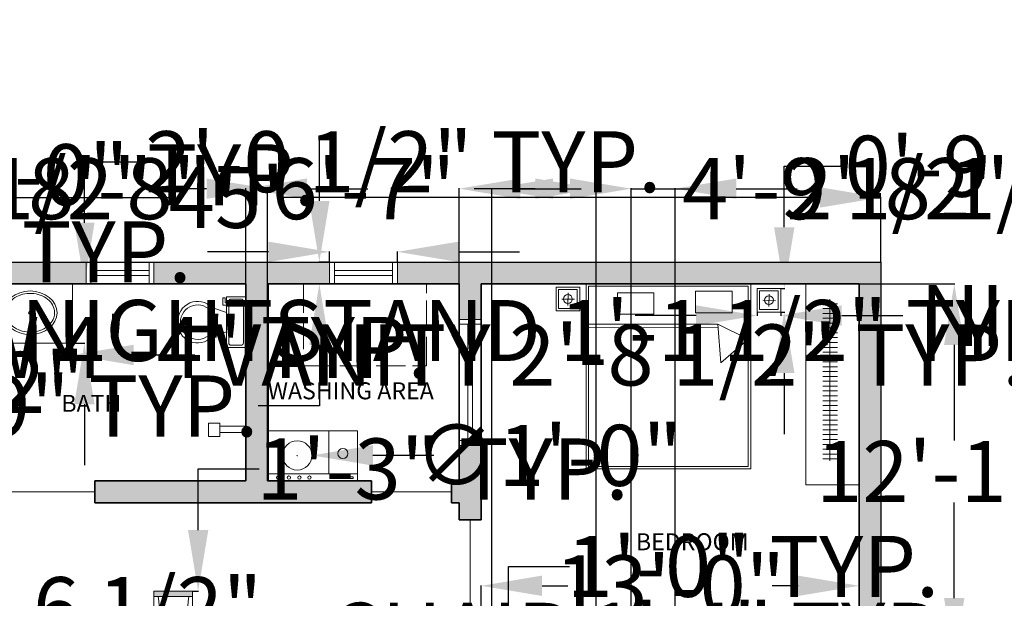
# Model space of a CAD drawing. Units: inches. Extents: x 29 to 6336, y 3 to 2592.
# Tile 7 of 8: x 5531 to 5938, y 2354 to 2592. Entities that reach past the tile are written whole.
import ezdxf

# ---------------------------------------------------------------- set-up
doc = ezdxf.new("R2010")
doc.units = ezdxf.units.IN
doc.header["$MEASUREMENT"] = 0
doc.linetypes.add('ACAD_ISO02W100', pattern=[15, 12, -3])
for name, color, linetype, lineweight in [('A-ANNO-DIMS', 2, 'Continuous', 18), ('A-AREA-IDEN', 7, 'Continuous', 18), ('A-DOOR', 4, 'Continuous', 18), ('A-EQPM', 9, 'Continuous', 18), ('A-EQPM-OVHD', 9, 'ACAD_ISO02W100', 13), ('A-FLOR-CASE', 8, 'Continuous', 18), ('A-FLOR-FIXT', 8, 'Continuous', 18), ('A-FURN', 8, 'Continuous', 18), ('A-GLAZ', 116, 'Continuous', 18), ('A-WALL', 7, 'Continuous', 35), ('A-WALL-PATT', 242, 'Continuous', 13), ('C-PROP', 7, 'Continuous', 25)]:
    doc.layers.add(name, color=color, linetype=linetype, lineweight=lineweight)
doc.styles.get("Standard").update_dxf_attribs({"font": 'arial.ttf'})
doc.dimstyles.get("Standard").update_dxf_attribs({"dimtxt": 25.18, "dimasz": 25.18, "dimexe": 0.18, "dimexo": 0.0625, "dimgap": 0.09, "dimtad": 0, "dimtih": 1, "dimtoh": 1, "dimdec": 0, "dimzin": 0, "dimdsep": 46, "dimlunit": 3, "dimtxsty": 'Standard', "dimcen": 0.09, "dimadec": 0, "dimazin": 0, "dimtfac": 1, "dimtdec": 0, "dimtofl": 0, "dimtmove": 0, "dimatfit": 3, "dimfxl": 1, "dimtolj": 1, "dimtzin": 0, "dimarcsym": 0})

# ---------------------------------------------------------------- blocks, each defined once
blk = doc.blocks.new('*U4')
for p, q in [((9.5, -6), (9.5, -2)), ((-8, -8.5), (-8, -8)), ((-7, -8), (-7, -9.5)), ((-4, -8), (-6, -14)), ((4, -8), (6, -14)), ((-10, -8.5), (-8, -8.5)), ((-10, -9.5), (-10, -8.5)), ((-7, -9.5), (-10, -9.5)), ((4, -14), (-4, -14))]:
    blk.add_line(p, q)
blk.add_lwpolyline([(10.5, -8), (10.5, 0), (-10.5, 0), (-10.5, -8)], close=True)
for points in [[(-9.5, -2), (-9.5, -6)], [(8.5, -1), (-8.5, -1)], [(-8.5, -7), (8.5, -7)]]:
    blk.add_lwpolyline(points)
for centre, radius, start, end in [((-8.625, -1.875), 0.8839, 81.8699, 188.1301), ((8.625, -1.875), 0.8839, 351.8699, 98.1301), ((-8.625, -6.125), 0.8839, 171.869898, 278.1301), ((8.625, -6.125), 0.8839, 261.8699, 8.1301), ((-0.4772, -19.9188), 8.0953, 133.01722, 273.38), ((0.0374, -19.8731), 7.127, 124.50543, 269.7), ((-0.0373, -19.8731), 7.127, 270.3, 55.4946), ((0.4773, -19.9188), 8.0953, 266.62, 46.9828)]:
    blk.add_arc(centre, radius, start, end)
blk = doc.blocks.new('*D5')
at = {"layer": 'A-ANNO-DIMS', "color": 0, "lineweight": -2, "transparency": 16777216}
for p, q in [((5346.66, 2492.39), (5346.66, 2519.15)), ((5371.84, 2518.97), (5594.69, 2518.97)), ((5861.48, 2518.97), (5638.62, 2518.97)), ((5886.66, 2492.39), (5886.66, 2519.15))]:
    blk.add_line(p, q, dxfattribs=at)
at = {"layer": 'A-ANNO-DIMS', "color": 0, "transparency": 16777216}
for points in [[(5371.84, 2523.17), (5371.84, 2514.77), (5346.66, 2518.97)], [(5861.48, 2523.17), (5861.48, 2514.77), (5886.66, 2518.97)]]:
    blk.add_solid(points, dxfattribs=at)
at = {"layer": 'Defpoints', "color": 0, "transparency": 16777216}
for p in [(5886.66, 2518.97), (5346.66, 2492.33), (5886.66, 2492.33)]:
    blk.add_point(p, dxfattribs=at)
at = {"layer": 'A-ANNO-DIMS', "color": 0, "transparency": 16777216, "insert": (5616.66, 2518.97), "char_height": 25.18, "attachment_point": 5}
blk.add_mtext("\\A1;45'", dxfattribs=at)
blk = doc.blocks.new('WIN-48')
for p, q in [((0, 9), (0, 0)), ((2, 9), (2, 0)), ((50, 9), (50, 0)), ((52, 9), (52, 0)), ((2, 5.5), (50, 5.5)), ((2, 3.5), (50, 3.5))]:
    blk.add_line(p, q)
blk = doc.blocks.new('WIN-24')
for p, q in [((0, 9), (0, 0)), ((2, 9), (2, 0)), ((26, 9), (26, 0)), ((28, 9), (28, 0)), ((2, 5.5), (26, 5.5)), ((2, 3.5), (26, 3.5))]:
    blk.add_line(p, q)
blk = doc.blocks.new('CHAIR-DINING')
h = blk.add_hatch(color=256)
h.dxf.hatch_style = 1
h.paths.add_polyline_path([(15.9, 12.75), (15.9, 15.02), (0, 15.02), (0, 12.75)])
for p, q in [((0, 0), (0, 15.02)), ((0, 15.02), (15.9, 15.02)), ((0, 12.75), (15.9, 12.75)), ((15.9, 15.02), (15.9, 0))]:
    blk.add_line(p, q)
for points in [[(1.75, 12.75), (2.84, 7.81), (1.97, 2.88), (1.75, 0)], [(14.44, 12.75), (13.78, 7.03), (13.63, 2.52), (14.44, 0)]]:
    blk.add_open_spline(points, degree=3)
blk = doc.blocks.new('NIGHTSTAND-10X10')
for p, q in [((2.31, 4.87), (7.57, 4.8)), ((4.94, 7.35), (4.88, 2.25))]:
    blk.add_line(p, q)
for points in [[(0, 9.74), (9.74, 9.74), (9.74, 0), (0, 0)], [(1, 8.74), (8.74, 8.74), (8.74, 1), (1, 1)]]:
    blk.add_lwpolyline(points, close=True)
blk.add_circle((4.87, 4.87), 1.82)
blk = doc.blocks.new('BASIN-VANITY')
for p, q in [((32.36, 0), (32.36, 24.47)), ((0, 0), (32.36, 0))]:
    blk.add_line(p, q)
blk.add_circle((14.85, 12.56), 0.667)
blk.add_ellipse((14.85, 12.56), major_axis=(11.1, 0), ratio=0.808824)
blk.add_open_spline([(24.95, 12.56), (24.95, 13.21), (24.85, 13.86), (24.35, 15.41), (23.86, 16.28), (22.49, 17.85), (21.62, 18.55), (19.61, 19.66), (18.47, 20.07), (16.07, 20.54), (14.82, 20.6), (12.37, 20.35), (11.18, 20.05), (9.01, 19.14), (8.04, 18.52), (6.44, 17.08), (5.81, 16.25), (4.97, 14.49), (4.75, 13.56), (4.73, 11.7), (4.93, 10.77), (5.73, 9), (6.33, 8.16), (7.89, 6.69), (8.85, 6.07), (10.99, 5.12), (12.18, 4.8), (14.62, 4.52), (15.88, 4.56), (18.29, 4.99), (19.44, 5.38), (21.47, 6.46), (22.36, 7.14), (23.77, 8.7), (24.29, 9.57), (24.83, 11.15), (24.95, 11.85), (24.95, 12.56)], degree=3, knots=[0, 0, 0, 0, 0.253102, 0.253102, 0.612978, 0.612978, 0.972853, 0.972853, 1.332728, 1.332728, 1.692603, 1.692603, 2.052478, 2.052478, 2.412354, 2.412354, 2.772229, 2.772229, 3.132104, 3.132104, 3.491979, 3.491979, 3.851854, 3.851854, 4.21173, 4.21173, 4.571605, 4.571605, 4.93148, 4.93148, 5.291355, 5.291355, 5.651231, 5.651231, 6.011106, 6.011106, 6.283185, 6.283185, 6.283185, 6.283185])
blk = doc.blocks.new('*D20')
at = {"layer": 'A-ANNO-DIMS', "color": 0, "lineweight": -2, "transparency": 16777216}
for p, q in [((5586.64, 2341.55), (5586.64, 2339.04)), ((5602.54, 2341.55), (5602.54, 2339.04)), ((5561.46, 2339.22), (5536.28, 2339.22)), ((5627.72, 2339.22), (5652.9, 2339.22))]:
    blk.add_line(p, q, dxfattribs=at)
at = {"layer": 'A-ANNO-DIMS', "color": 0, "transparency": 16777216}
for points in [[(5561.46, 2343.42), (5561.46, 2335.03), (5586.64, 2339.22)], [(5627.72, 2343.42), (5627.72, 2335.03), (5602.54, 2339.22)]]:
    blk.add_solid(points, dxfattribs=at)
at = {"layer": 'Defpoints', "color": 0, "transparency": 16777216}
for p in [(5586.64, 2341.61), (5602.54, 2341.61), (5602.54, 2339.22)]:
    blk.add_point(p, dxfattribs=at)
at = {"layer": 'A-ANNO-DIMS', "color": 0, "transparency": 16777216, "insert": (5789.2, 2339.22), "char_height": 25.18, "attachment_point": 5}
blk.add_mtext('\\A1;CHAIR 1\'-4" TYP.', dxfattribs=at)
blk = doc.blocks.new('*D21')
at = {"layer": 'A-ANNO-DIMS', "color": 0, "lineweight": -2, "transparency": 16777216}
for p, q in [((5604.93, 2381.81), (5604.93, 2406.99)), ((5604.93, 2406.99), (5630.11, 2406.99)), ((5602.6, 2356.63), (5605.11, 2356.63)), ((5602.6, 2341.61), (5605.11, 2341.61)), ((5604.93, 2316.43), (5604.93, 2291.25))]:
    blk.add_line(p, q, dxfattribs=at)
at = {"layer": 'A-ANNO-DIMS', "color": 0, "transparency": 16777216}
for points in [[(5600.73, 2381.81), (5609.12, 2381.81), (5604.93, 2356.63)], [(5600.73, 2316.43), (5609.12, 2316.43), (5604.93, 2341.61)]]:
    blk.add_solid(points, dxfattribs=at)
at = {"layer": 'Defpoints', "color": 0, "transparency": 16777216}
for p in [(5602.54, 2356.63), (5604.93, 2356.63), (5602.54, 2341.61)]:
    blk.add_point(p, dxfattribs=at)
at = {"layer": 'A-ANNO-DIMS', "color": 0, "transparency": 16777216, "insert": (5705.75, 2406.99), "char_height": 25.18, "attachment_point": 5}
blk.add_mtext('\\A1;1\'-3" TYP.', dxfattribs=at)
blk = doc.blocks.new('*D22')
at = {"layer": 'A-ANNO-DIMS', "color": 0, "lineweight": -2, "transparency": 16777216}
for p, q in [((5363.46, 2431.95), (5363.46, 2457.13)), ((5363.46, 2457.13), (5388.64, 2457.13)), ((5355.72, 2431.95), (5363.64, 2431.95)), ((5363.46, 2405.13), (5363.46, 2406.77)), ((5355.72, 2379.95), (5363.64, 2379.95))]:
    blk.add_line(p, q, dxfattribs=at)
at = {"layer": 'A-ANNO-DIMS', "color": 0, "transparency": 16777216}
for points in [[(5359.26, 2406.77), (5367.65, 2406.77), (5363.46, 2431.95)], [(5359.26, 2405.13), (5367.65, 2405.13), (5363.46, 2379.95)]]:
    blk.add_solid(points, dxfattribs=at)
at = {"layer": 'Defpoints', "color": 0, "transparency": 16777216}
for p in [(5355.66, 2431.95), (5363.46, 2431.95), (5355.66, 2379.95)]:
    blk.add_point(p, dxfattribs=at)
at = {"layer": 'A-ANNO-DIMS', "color": 0, "transparency": 16777216, "insert": (5548.04, 2457.13), "char_height": 25.18, "attachment_point": 5}
blk.add_mtext('\\A1;WINDOW 4\'-4" TYP.', dxfattribs=at)
blk = doc.blocks.new('*D26')
at = {"layer": 'A-ANNO-DIMS', "color": 0, "lineweight": -2, "transparency": 16777216}
for p, q in [((5633.95, 2496.53), (5608.77, 2496.53)), ((5659.13, 2492.39), (5659.13, 2496.71)), ((5687.13, 2492.39), (5687.13, 2496.71)), ((5712.31, 2496.53), (5737.49, 2496.53))]:
    blk.add_line(p, q, dxfattribs=at)
at = {"layer": 'A-ANNO-DIMS', "color": 0, "transparency": 16777216}
for points in [[(5633.95, 2500.73), (5633.95, 2492.33), (5659.13, 2496.53)], [(5712.31, 2500.73), (5712.31, 2492.33), (5687.13, 2496.53)]]:
    blk.add_solid(points, dxfattribs=at)
at = {"layer": 'Defpoints', "color": 0, "transparency": 16777216}
for p in [(5659.13, 2496.53), (5659.13, 2492.33), (5687.13, 2492.33)]:
    blk.add_point(p, dxfattribs=at)
at = {"layer": 'A-ANNO-DIMS', "color": 0, "transparency": 16777216, "insert": (5449.36, 2496.53), "char_height": 25.18, "attachment_point": 5}
blk.add_mtext('\\A1;WINDOW 2\'-4" TYP.', dxfattribs=at)
blk = doc.blocks.new('*D27')
at = {"layer": 'A-ANNO-DIMS', "color": 0, "lineweight": -2, "transparency": 16777216}
for p, q in [((5654.93, 2517.51), (5654.93, 2542.69)), ((5659.07, 2492.33), (5654.75, 2492.33)), ((5659.07, 2483.33), (5654.75, 2483.33)), ((5654.93, 2458.15), (5654.93, 2432.97)), ((5654.93, 2432.97), (5629.75, 2432.97))]:
    blk.add_line(p, q, dxfattribs=at)
at = {"layer": 'A-ANNO-DIMS', "color": 0, "transparency": 16777216}
for points in [[(5650.73, 2517.51), (5659.12, 2517.51), (5654.93, 2492.33)], [(5650.73, 2458.15), (5659.12, 2458.15), (5654.93, 2483.33)]]:
    blk.add_solid(points, dxfattribs=at)
at = {"layer": 'Defpoints', "color": 0, "transparency": 16777216}
for p in [(5659.13, 2492.33), (5654.93, 2483.33), (5659.13, 2483.33)]:
    blk.add_point(p, dxfattribs=at)
at = {"layer": 'A-ANNO-DIMS', "color": 0, "transparency": 16777216, "insert": (5552.92, 2432.97), "char_height": 25.18, "attachment_point": 5}
blk.add_mtext('\\A1;0\'-9" TYP.', dxfattribs=at)
blk = doc.blocks.new('*D30')
at = {"layer": 'A-ANNO-DIMS', "color": 0, "lineweight": -2, "transparency": 16777216}
for p, q in [((5810.39, 2470.26), (5785.21, 2470.26)), ((5835.57, 2471.66), (5835.57, 2470.08)), ((5845.31, 2471.66), (5845.31, 2470.08)), ((5870.49, 2470.26), (5895.67, 2470.26))]:
    blk.add_line(p, q, dxfattribs=at)
at = {"layer": 'A-ANNO-DIMS', "color": 0, "transparency": 16777216}
for points in [[(5810.39, 2474.46), (5810.39, 2466.06), (5835.57, 2470.26)], [(5870.49, 2474.46), (5870.49, 2466.06), (5845.31, 2470.26)]]:
    blk.add_solid(points, dxfattribs=at)
at = {"layer": 'Defpoints', "color": 0, "transparency": 16777216}
for p in [(5835.57, 2471.72), (5845.31, 2471.72), (5845.31, 2470.26)]:
    blk.add_point(p, dxfattribs=at)
at = {"layer": 'A-ANNO-DIMS', "color": 0, "transparency": 16777216, "insert": (6120.44, 2470.26), "char_height": 25.18, "attachment_point": 5}
blk.add_mtext('\\A1;NIGHTSTAND 0\'-9 1/2" TYP.', dxfattribs=at)
blk = doc.blocks.new('*D31')
at = {"layer": 'A-ANNO-DIMS', "color": 0, "lineweight": -2, "transparency": 16777216}
for p, q in [((5846.78, 2506.64), (5846.78, 2531.82)), ((5846.78, 2531.82), (5871.96, 2531.82)), ((5845.38, 2481.46), (5846.96, 2481.46)), ((5845.38, 2471.72), (5846.96, 2471.72)), ((5846.78, 2446.54), (5846.78, 2421.36))]:
    blk.add_line(p, q, dxfattribs=at)
at = {"layer": 'A-ANNO-DIMS', "color": 0, "transparency": 16777216}
for points in [[(5842.58, 2506.64), (5850.97, 2506.64), (5846.78, 2481.46)], [(5842.58, 2446.54), (5850.97, 2446.54), (5846.78, 2471.72)]]:
    blk.add_solid(points, dxfattribs=at)
at = {"layer": 'Defpoints', "color": 0, "transparency": 16777216}
for p in [(5845.31, 2481.46), (5846.78, 2481.46), (5845.31, 2471.72)]:
    blk.add_point(p, dxfattribs=at)
at = {"layer": 'A-ANNO-DIMS', "color": 0, "transparency": 16777216, "insert": (5978.13, 2531.82), "char_height": 25.18, "attachment_point": 5}
blk.add_mtext('\\A1;0\'-9 1/2" TYP.', dxfattribs=at)
blk = doc.blocks.new('*D32')
at = {"layer": 'A-ANNO-DIMS', "color": 0, "lineweight": -2, "transparency": 16777216}
for p, q in [((5709.84, 2318.47), (5684.66, 2318.47)), ((5735.02, 2316.52), (5735.02, 2318.65)), ((5748.43, 2316.52), (5748.43, 2318.65)), ((5773.61, 2318.47), (5798.79, 2318.47))]:
    blk.add_line(p, q, dxfattribs=at)
at = {"layer": 'A-ANNO-DIMS', "color": 0, "transparency": 16777216}
for points in [[(5709.84, 2322.67), (5709.84, 2314.27), (5735.02, 2318.47)], [(5773.61, 2322.67), (5773.61, 2314.27), (5748.43, 2318.47)]]:
    blk.add_solid(points, dxfattribs=at)
at = {"layer": 'Defpoints', "color": 0, "transparency": 16777216}
for p in [(5735.02, 2316.46), (5748.43, 2318.47), (5748.43, 2316.46)]:
    blk.add_point(p, dxfattribs=at)
at = {"layer": 'A-ANNO-DIMS', "color": 0, "transparency": 16777216, "insert": (6023.56, 2318.47), "char_height": 25.18, "attachment_point": 5}
blk.add_mtext('\\A1;NIGHTSTAND 1\'-1 1/2" TYP.', dxfattribs=at)
blk = doc.blocks.new('*D33')
at = {"layer": 'A-ANNO-DIMS', "color": 0, "lineweight": -2, "transparency": 16777216}
for p, q in [((5733.01, 2341.64), (5733.01, 2366.82)), ((5733.01, 2366.82), (5758.19, 2366.82)), ((5734.96, 2316.46), (5732.83, 2316.46)), ((5734.96, 2304.36), (5732.83, 2304.36)), ((5733.01, 2279.18), (5733.01, 2254))]:
    blk.add_line(p, q, dxfattribs=at)
at = {"layer": 'A-ANNO-DIMS', "color": 0, "transparency": 16777216}
for points in [[(5728.81, 2341.64), (5737.21, 2341.64), (5733.01, 2316.46)], [(5728.81, 2279.18), (5737.21, 2279.18), (5733.01, 2304.36)]]:
    blk.add_solid(points, dxfattribs=at)
at = {"layer": 'Defpoints', "color": 0, "transparency": 16777216}
for p in [(5733.01, 2316.46), (5735.02, 2316.46), (5735.02, 2304.36)]:
    blk.add_point(p, dxfattribs=at)
at = {"layer": 'A-ANNO-DIMS', "color": 0, "transparency": 16777216, "insert": (5833.84, 2366.82), "char_height": 25.18, "attachment_point": 5}
blk.add_mtext('\\A1;1\'-0" TYP.', dxfattribs=at)
blk = doc.blocks.new('*D36')
at = {"layer": 'A-ANNO-DIMS', "color": 0, "lineweight": -2, "transparency": 16777216}
for p, q in [((5520.77, 2458.79), (5520.77, 2453.82)), ((5553.13, 2458.79), (5553.13, 2453.82)), ((5495.59, 2454), (5470.41, 2454)), ((5578.31, 2454), (5603.49, 2454))]:
    blk.add_line(p, q, dxfattribs=at)
at = {"layer": 'A-ANNO-DIMS', "color": 0, "transparency": 16777216}
for points in [[(5495.59, 2458.2), (5495.59, 2449.81), (5520.77, 2454)], [(5578.31, 2458.2), (5578.31, 2449.81), (5553.13, 2454)]]:
    blk.add_solid(points, dxfattribs=at)
at = {"layer": 'Defpoints', "color": 0, "transparency": 16777216}
for p in [(5520.77, 2458.86), (5553.13, 2458.86), (5553.13, 2454)]:
    blk.add_point(p, dxfattribs=at)
at = {"layer": 'A-ANNO-DIMS', "color": 0, "transparency": 16777216, "insert": (5778.73, 2454), "char_height": 25.18, "attachment_point": 5}
blk.add_mtext('\\A1;VANITY 2\'-8 1/2" TYP.', dxfattribs=at)
blk = doc.blocks.new('*D37')
at = {"layer": 'A-ANNO-DIMS', "color": 0, "lineweight": -2, "transparency": 16777216}
for p, q in [((5557.99, 2508.51), (5557.99, 2533.69)), ((5557.99, 2533.69), (5583.17, 2533.69)), ((5553.2, 2483.33), (5558.17, 2483.33)), ((5553.2, 2458.86), (5558.17, 2458.86)), ((5557.99, 2433.68), (5557.99, 2408.5))]:
    blk.add_line(p, q, dxfattribs=at)
at = {"layer": 'A-ANNO-DIMS', "color": 0, "transparency": 16777216}
for points in [[(5553.79, 2508.51), (5562.18, 2508.51), (5557.99, 2483.33)], [(5553.79, 2433.68), (5562.18, 2433.68), (5557.99, 2458.86)]]:
    blk.add_solid(points, dxfattribs=at)
at = {"layer": 'Defpoints', "color": 0, "transparency": 16777216}
for p in [(5553.13, 2483.33), (5557.99, 2483.33), (5553.13, 2458.86)]:
    blk.add_point(p, dxfattribs=at)
at = {"layer": 'A-ANNO-DIMS', "color": 0, "transparency": 16777216, "insert": (5689.55, 2533.69), "char_height": 25.18, "attachment_point": 5}
blk.add_mtext('\\A1;2\'-0 1/2" TYP.', dxfattribs=at)
blk = doc.blocks.new('*D40')
at = {"layer": 'A-ANNO-DIMS', "color": 0, "lineweight": -2, "transparency": 16777216}
for p, q in [((5460.58, 2466.07), (5460.58, 2463.89)), ((5474.29, 2466.07), (5474.29, 2463.89)), ((5435.4, 2464.07), (5410.22, 2464.07)), ((5499.47, 2464.07), (5524.65, 2464.07))]:
    blk.add_line(p, q, dxfattribs=at)
at = {"layer": 'A-ANNO-DIMS', "color": 0, "transparency": 16777216}
for points in [[(5435.4, 2468.27), (5435.4, 2459.88), (5460.58, 2464.07)], [(5499.47, 2468.27), (5499.47, 2459.88), (5474.29, 2464.07)]]:
    blk.add_solid(points, dxfattribs=at)
at = {"layer": 'Defpoints', "color": 0, "transparency": 16777216}
for p in [(5460.58, 2466.13), (5474.29, 2466.13), (5474.29, 2464.07)]:
    blk.add_point(p, dxfattribs=at)
at = {"layer": 'A-ANNO-DIMS', "color": 0, "transparency": 16777216, "insert": (5749.42, 2464.07), "char_height": 25.18, "attachment_point": 5}
blk.add_mtext('\\A1;NIGHTSTAND 1\'-1 1/2" TYP.', dxfattribs=at)
blk = doc.blocks.new('*D41')
at = {"layer": 'A-ANNO-DIMS', "color": 0, "lineweight": -2, "transparency": 16777216}
for p, q in [((5476.35, 2503.16), (5476.35, 2528.34)), ((5476.35, 2528.34), (5501.53, 2528.34)), ((5474.36, 2477.98), (5476.53, 2477.98)), ((5474.36, 2466.13), (5476.53, 2466.13)), ((5476.35, 2440.95), (5476.35, 2415.77))]:
    blk.add_line(p, q, dxfattribs=at)
at = {"layer": 'A-ANNO-DIMS', "color": 0, "transparency": 16777216}
for points in [[(5472.16, 2503.16), (5480.55, 2503.16), (5476.35, 2477.98)], [(5472.16, 2440.95), (5480.55, 2440.95), (5476.35, 2466.13)]]:
    blk.add_solid(points, dxfattribs=at)
at = {"layer": 'Defpoints', "color": 0, "transparency": 16777216}
for p in [(5474.29, 2477.98), (5476.35, 2477.98), (5474.29, 2466.13)]:
    blk.add_point(p, dxfattribs=at)
at = {"layer": 'A-ANNO-DIMS', "color": 0, "transparency": 16777216, "insert": (5577.18, 2528.34), "char_height": 25.18, "attachment_point": 5}
blk.add_mtext('\\A1;1\'-0" TYP.', dxfattribs=at)
blk = doc.blocks.new('*D43')
at = {"layer": 'A-ANNO-DIMS', "color": 0, "lineweight": -2, "transparency": 16777216}
for p, q in [((5495.59, 2522.58), (5470.41, 2522.58)), ((5520.77, 2483.39), (5520.77, 2522.76)), ((5624.6, 2483.39), (5624.6, 2522.76)), ((5649.78, 2522.58), (5674.96, 2522.58))]:
    blk.add_line(p, q, dxfattribs=at)
at = {"layer": 'A-ANNO-DIMS', "color": 0, "transparency": 16777216}
for points in [[(5495.59, 2526.78), (5495.59, 2518.38), (5520.77, 2522.58)], [(5649.78, 2526.78), (5649.78, 2518.38), (5624.6, 2522.58)]]:
    blk.add_solid(points, dxfattribs=at)
at = {"layer": 'Defpoints', "color": 0, "transparency": 16777216}
for p in [(5624.6, 2522.58), (5520.77, 2483.33), (5624.6, 2483.33)]:
    blk.add_point(p, dxfattribs=at)
at = {"layer": 'A-ANNO-DIMS', "color": 0, "transparency": 16777216, "insert": (5572.68, 2522.58), "char_height": 25.18, "attachment_point": 5}
blk.add_mtext('\\A1;8\'-8"', dxfattribs=at)
blk = doc.blocks.new('*D44')
at = {"layer": 'A-ANNO-DIMS', "color": 0, "lineweight": -2, "transparency": 16777216}
for p, q in [((5608.42, 2522.58), (5583.24, 2522.58)), ((5633.6, 2483.39), (5633.6, 2522.76)), ((5712.66, 2483.39), (5712.66, 2522.76)), ((5737.84, 2522.58), (5763.02, 2522.58))]:
    blk.add_line(p, q, dxfattribs=at)
at = {"layer": 'A-ANNO-DIMS', "color": 0, "transparency": 16777216}
for points in [[(5608.42, 2526.78), (5608.42, 2518.38), (5633.6, 2522.58)], [(5737.84, 2526.78), (5737.84, 2518.38), (5712.66, 2522.58)]]:
    blk.add_solid(points, dxfattribs=at)
at = {"layer": 'Defpoints', "color": 0, "transparency": 16777216}
for p in [(5712.66, 2522.58), (5633.6, 2483.33), (5712.66, 2483.33)]:
    blk.add_point(p, dxfattribs=at)
at = {"layer": 'A-ANNO-DIMS', "color": 0, "transparency": 16777216, "insert": (5673.13, 2522.58), "char_height": 25.18, "attachment_point": 5}
blk.add_mtext('\\A1;6\'-7"', dxfattribs=at)
blk = doc.blocks.new('*D45')
at = {"layer": 'A-ANNO-DIMS', "color": 0, "lineweight": -2, "transparency": 16777216}
for p, q in [((5721.66, 2328.63), (5721.66, 2358.99)), ((5746.84, 2358.81), (5757.5, 2358.81)), ((5852.48, 2358.81), (5841.81, 2358.81)), ((5877.66, 2328.63), (5877.66, 2358.99))]:
    blk.add_line(p, q, dxfattribs=at)
at = {"layer": 'A-ANNO-DIMS', "color": 0, "transparency": 16777216}
for points in [[(5746.84, 2363.01), (5746.84, 2354.62), (5721.66, 2358.81)], [(5852.48, 2363.01), (5852.48, 2354.62), (5877.66, 2358.81)]]:
    blk.add_solid(points, dxfattribs=at)
at = {"layer": 'Defpoints', "color": 0, "transparency": 16777216}
for p in [(5877.66, 2358.81), (5721.66, 2328.56), (5877.66, 2328.56)]:
    blk.add_point(p, dxfattribs=at)
at = {"layer": 'A-ANNO-DIMS', "color": 0, "transparency": 16777216, "insert": (5799.66, 2358.81), "char_height": 25.18, "attachment_point": 5}
blk.add_mtext('\\A1;13\'-0"', dxfattribs=at)
blk = doc.blocks.new('*D46')
at = {"layer": 'A-ANNO-DIMS', "color": 0, "lineweight": -2, "transparency": 16777216}
for p, q in [((5877.72, 2483.33), (5917.09, 2483.33)), ((5916.91, 2458.15), (5916.91, 2418.68)), ((5916.91, 2353.74), (5916.91, 2393.21)), ((5877.72, 2328.56), (5917.09, 2328.56))]:
    blk.add_line(p, q, dxfattribs=at)
at = {"layer": 'A-ANNO-DIMS', "color": 0, "transparency": 16777216}
for points in [[(5912.71, 2458.15), (5921.1, 2458.15), (5916.91, 2483.33)], [(5912.71, 2353.74), (5921.1, 2353.74), (5916.91, 2328.56)]]:
    blk.add_solid(points, dxfattribs=at)
at = {"layer": 'Defpoints', "color": 0, "transparency": 16777216}
for p in [(5877.66, 2483.33), (5916.91, 2483.33), (5877.66, 2328.56)]:
    blk.add_point(p, dxfattribs=at)
at = {"layer": 'A-ANNO-DIMS', "color": 0, "transparency": 16777216, "insert": (5916.91, 2405.95), "char_height": 25.18, "attachment_point": 5}
blk.add_mtext('\\A1;12\'-11"', dxfattribs=at)
blk = doc.blocks.new('*D47')
at = {"layer": 'A-ANNO-DIMS', "color": 0, "lineweight": -2, "transparency": 16777216}
for p, q in [((5520.71, 2483.33), (5490.34, 2483.33)), ((5490.52, 2458.15), (5490.52, 2455.8)), ((5490.52, 2427.23), (5490.52, 2429.58)), ((5520.71, 2402.05), (5490.34, 2402.05))]:
    blk.add_line(p, q, dxfattribs=at)
at = {"layer": 'A-ANNO-DIMS', "color": 0, "transparency": 16777216}
for points in [[(5486.32, 2458.15), (5494.72, 2458.15), (5490.52, 2483.33)], [(5486.32, 2427.23), (5494.72, 2427.23), (5490.52, 2402.05)]]:
    blk.add_solid(points, dxfattribs=at)
at = {"layer": 'Defpoints', "color": 0, "transparency": 16777216}
for p in [(5490.52, 2483.33), (5520.77, 2483.33), (5520.77, 2402.05)]:
    blk.add_point(p, dxfattribs=at)
at = {"layer": 'A-ANNO-DIMS', "color": 0, "transparency": 16777216, "insert": (5490.52, 2442.69), "char_height": 25.18, "attachment_point": 5}
blk.add_mtext('\\A1;6\'-9 1/2"', dxfattribs=at)
blk = doc.blocks.new('*D48')
at = {"layer": 'A-ANNO-DIMS', "color": 0, "lineweight": -2, "transparency": 16777216}
for p, q in [((5351.16, 2319.63), (5351.16, 2522.76)), ((5376.34, 2522.58), (5385.42, 2522.58)), ((5410.6, 2319.63), (5410.6, 2522.76)), ((5410.6, 2522.58), (5435.78, 2522.58))]:
    blk.add_line(p, q, dxfattribs=at)
at = {"layer": 'A-ANNO-DIMS', "color": 0, "transparency": 16777216}
for points in [[(5376.34, 2526.78), (5376.34, 2518.38), (5351.16, 2522.58)], [(5385.42, 2526.78), (5385.42, 2518.38), (5410.6, 2522.58)]]:
    blk.add_solid(points, dxfattribs=at)
at = {"layer": 'Defpoints', "color": 0, "transparency": 16777216}
for p in [(5410.6, 2522.58), (5351.16, 2319.56), (5410.6, 2319.56)]:
    blk.add_point(p, dxfattribs=at)
at = {"layer": 'A-ANNO-DIMS', "color": 0, "transparency": 16777216, "insert": (5508.96, 2522.58), "char_height": 25.18, "attachment_point": 5}
blk.add_mtext('\\A1;4\'-11 1/2"', dxfattribs=at)
blk = doc.blocks.new('*D65')
at = {"layer": 'A-ANNO-DIMS', "color": 0, "lineweight": -2, "transparency": 16777216}
for p, q in [((5726.12, 2182.71), (5726.12, 2522.76)), ((5751.3, 2522.58), (5758.41, 2522.58)), ((5783.59, 2182.71), (5783.59, 2522.76)), ((5783.59, 2522.58), (5808.77, 2522.58))]:
    blk.add_line(p, q, dxfattribs=at)
at = {"layer": 'A-ANNO-DIMS', "color": 0, "transparency": 16777216}
for points in [[(5751.3, 2526.78), (5751.3, 2518.38), (5726.12, 2522.58)], [(5758.41, 2526.78), (5758.41, 2518.38), (5783.59, 2522.58)]]:
    blk.add_solid(points, dxfattribs=at)
at = {"layer": 'Defpoints', "color": 0, "transparency": 16777216}
for p in [(5783.59, 2522.58), (5726.12, 2182.65), (5783.59, 2182.65)]:
    blk.add_point(p, dxfattribs=at)
at = {"layer": 'A-ANNO-DIMS', "color": 0, "transparency": 16777216, "insert": (5872.17, 2522.58), "char_height": 25.18, "attachment_point": 5}
blk.add_mtext('\\A1;4\'-9 1/2"', dxfattribs=at)
blk = doc.blocks.new('*D67')
at = {"layer": 'A-ANNO-DIMS', "color": 0, "lineweight": -2, "transparency": 16777216}
for p, q in [((5743.99, 2522.58), (5718.81, 2522.58)), ((5769.17, 2150.03), (5769.17, 2522.76)), ((5801.76, 2182.71), (5801.76, 2522.76)), ((5826.94, 2522.58), (5852.12, 2522.58))]:
    blk.add_line(p, q, dxfattribs=at)
at = {"layer": 'A-ANNO-DIMS', "color": 0, "transparency": 16777216}
for points in [[(5743.99, 2526.78), (5743.99, 2518.38), (5769.17, 2522.58)], [(5826.94, 2526.78), (5826.94, 2518.38), (5801.76, 2522.58)]]:
    blk.add_solid(points, dxfattribs=at)
at = {"layer": 'Defpoints', "color": 0, "transparency": 16777216}
for p in [(5801.76, 2522.58), (5801.76, 2182.65), (5769.17, 2149.97)]:
    blk.add_point(p, dxfattribs=at)
at = {"layer": 'A-ANNO-DIMS', "color": 0, "transparency": 16777216, "insert": (5915.23, 2522.58), "char_height": 25.18, "attachment_point": 5}
blk.add_mtext('\\A1;2\'-8 1/2"', dxfattribs=at)
blk = doc.blocks.new('*D69')
at = {"layer": 'A-ANNO-DIMS', "color": 0, "lineweight": -2, "transparency": 16777216}
for p, q in [((5394.42, 2349.81), (5369.24, 2349.81)), ((5419.6, 2319.63), (5419.6, 2349.99)), ((5450.34, 2319.63), (5450.34, 2349.99)), ((5475.52, 2349.81), (5500.7, 2349.81))]:
    blk.add_line(p, q, dxfattribs=at)
at = {"layer": 'A-ANNO-DIMS', "color": 0, "transparency": 16777216}
for points in [[(5394.42, 2354.01), (5394.42, 2345.62), (5419.6, 2349.81)], [(5475.52, 2354.01), (5475.52, 2345.62), (5450.34, 2349.81)]]:
    blk.add_solid(points, dxfattribs=at)
at = {"layer": 'Defpoints', "color": 0, "transparency": 16777216}
for p in [(5450.34, 2349.81), (5419.6, 2319.56), (5450.34, 2319.56)]:
    blk.add_point(p, dxfattribs=at)
at = {"layer": 'A-ANNO-DIMS', "color": 0, "transparency": 16777216, "insert": (5563.81, 2349.81), "char_height": 25.18, "attachment_point": 5}
blk.add_mtext('\\A1;2\'-6 1/2"', dxfattribs=at)
blk = doc.blocks.new('*D72')
at = {"layer": 'A-ANNO-DIMS', "color": 0, "lineweight": -2, "transparency": 16777216}
for p, q in [((5645.73, 2412.58), (5645.91, 2412.58)), ((5645.82, 2412.49), (5645.82, 2412.67)), ((5702.23, 2412.59), (5677.05, 2412.59))]:
    blk.add_line(p, q, dxfattribs=at)
at = {"layer": 'A-ANNO-DIMS', "color": 0, "transparency": 16777216}
blk.add_solid([(5677.05, 2416.78), (5677.05, 2408.39), (5651.87, 2412.59)], dxfattribs=at)
at = {"layer": 'Defpoints', "color": 0, "transparency": 16777216}
for p in [(5639.77, 2412.58), (5651.87, 2412.59)]:
    blk.add_point(p, dxfattribs=at)
at = {"layer": 'A-ANNO-DIMS', "color": 0, "transparency": 16777216, "insert": (5749.49, 2412.59), "char_height": 25.18, "attachment_point": 5}
blk.add_mtext('\\A1;∅1\'-0"', dxfattribs=at)

msp = doc.modelspace()

# ---------------------------------------------------------------- hatches: boundary and pattern name
at = {"layer": 'A-WALL-PATT'}
h = msp.add_hatch(color=256, dxfattribs=at)
h.dxf.hatch_style = 1
h.paths.add_polyline_path([(5558.68, 2492.33), (5459.71, 2492.33), (5459.71, 2483.33), (5511.77, 2483.33), (5511.77, 2388.68), (5520.77, 2388.68), (5520.77, 2393.05), (5526.31, 2393.05), (5526.31, 2402.05), (5520.77, 2402.05), (5520.77, 2483.33), (5558.68, 2483.33)])
h.paths.add_polyline_path([(5659.13, 2492.33), (5586.68, 2492.33), (5586.68, 2483.33), (5624.6, 2483.33), (5624.6, 2402.05), (5562.29, 2402.05), (5562.29, 2393.05), (5676.48, 2393.05), (5676.48, 2402.05), (5633.6, 2402.05), (5633.6, 2422.71), (5633.6, 2483.33), (5659.13, 2483.33)])
h.paths.add_polyline_path([(5886.66, 2492.33), (5687.13, 2492.33), (5687.13, 2483.33), (5712.66, 2483.33), (5712.66, 2468.69), (5721.66, 2468.69), (5721.66, 2483.33), (5877.66, 2483.33), (5877.66, 2106.48), (5858.21, 2106.48), (5858.21, 2097.48), (5877.66, 2097.48), (5877.66, 1961.33), (5877.66, 1952.33), (5886.66, 1952.33)])
h.paths.add_polyline_path([(5721.66, 2416.69), (5712.66, 2416.69), (5712.66, 2402.05), (5709.45, 2402.05), (5709.45, 2393.05), (5712.66, 2393.05), (5712.66, 2386.01), (5721.66, 2386.01)], flags=17)
h.paths.add_polyline_path([(5355.66, 2483.33), (5407.71, 2483.33), (5407.71, 2492.33), (5346.66, 2492.33), (5346.66, 2431.95), (5355.66, 2431.95)])
h.paths.add_polyline_path([(5355.66, 2379.95), (5346.66, 2379.95), (5346.66, 2319.56), (5355.66, 2319.56), (5355.66, 2328.56)])
h.paths.add_polyline_path([(5520.77, 2337.13), (5511.77, 2337.13), (5511.77, 2328.56), (5410.6, 2328.56), (5410.6, 2319.56), (5410.6, 2281.61), (5419.6, 2281.61), (5419.6, 2319.56), (5510.11, 2319.56), (5510.11, 2234.67), (5519.11, 2234.67), (5519.11, 2319.56), (5520.77, 2319.56)])
h.paths.add_polyline_path([(5519.11, 2197.33), (5510.11, 2197.33), (5510.11, 2191.65), (5419.6, 2191.65), (5419.6, 2228.6), (5419.6, 2229.61), (5410.6, 2229.61), (5410.6, 2182.65), (5519.11, 2182.65)])
h.paths.add_polyline_path([(5712.66, 2193.6), (5592.36, 2193.6), (5592.36, 2182.65), (5624.77, 2182.65), (5633.77, 2182.65), (5712.66, 2182.65)])
h.paths.add_polyline_path([(5633.77, 2182.65), (5624.77, 2182.65), (5624.77, 2051.72), (5633.77, 2051.72), (5691.77, 2051.72), (5691.77, 2060.72), (5633.77, 2060.72)])
h.paths.add_polyline_path([(5810.76, 2097.48), (5830.21, 2097.48), (5830.21, 2106.48), (5810.76, 2106.48), (5810.76, 2182.65), (5817.87, 2182.65), (5817.87, 2193.6), (5783.59, 2193.6), (5783.59, 2182.65), (5801.76, 2182.65), (5801.76, 2060.72), (5743.77, 2060.72), (5743.77, 2051.72), (5810.76, 2051.72)], flags=17)
h.paths.add_polyline_path([(5721.66, 2319.56), (5877.66, 2319.56), (5877.66, 2328.56), (5721.66, 2328.56), (5721.66, 2335.85), (5712.66, 2335.85), (5712.66, 2319.56), (5712.66, 2182.65), (5726.12, 2182.65), (5726.12, 2193.6), (5721.66, 2193.6)], flags=17)
h.paths.add_polyline_path([(5631.73, 2431.78), (5711.31, 2431.78), (5711.31, 2446.2), (5631.73, 2446.2)], flags=9)

# ---------------------------------------------------------------- linework, layer by layer
at = {"layer": 'A-DOOR'}
for p, q in [((5526.31, 2397.55), (5562.29, 2397.55)), ((5676.48, 2397.55), (5709.45, 2397.55)), ((5717.16, 2386.01), (5717.16, 2335.85))]:
    msp.add_line(p, q, dxfattribs=at)
at = {"layer": 'A-EQPM'}
for p, q in [((5658.78, 2422.71), (5658.78, 2405)), ((5633.77, 2405), (5670.61, 2405))]:
    msp.add_line(p, q, dxfattribs=at)
for points in [[(5633.6, 2402.05), (5670.61, 2402.05), (5670.61, 2422.71), (5633.6, 2422.71)], [(5660.24, 2403.78), (5668.84, 2403.78), (5668.84, 2403.03), (5660.24, 2403.03)]]:
    msp.add_lwpolyline(points, close=True, dxfattribs=at)
for centre, radius in [((5645.82, 2412.58), 6.05), ((5664.67, 2413.36), 2.07), ((5637.9, 2403.41), 0.689), ((5642.36, 2403.41), 0.689), ((5646.69, 2403.41), 0.689), ((5650.83, 2403.41), 0.689)]:
    msp.add_circle(centre, radius, dxfattribs=at)
at = {"layer": 'A-EQPM-OVHD'}
for p, q in [((5648.43, 2483.33), (5648.43, 2449.49)), ((5699.18, 2449.49), (5699.18, 2483.33)), ((5648.43, 2449.49), (5699.18, 2449.49))]:
    msp.add_line(p, q, dxfattribs=at)
at = {"layer": 'A-FLOR-CASE'}
for p, q in [((5855.72, 2483.33), (5855.72, 2400.5)), ((5862.66, 2475.15), (5868.71, 2475.15)), ((5865.63, 2477.06), (5865.63, 2410.34)), ((5862.66, 2473.15), (5868.71, 2473.15)), ((5862.66, 2471.15), (5868.71, 2471.15)), ((5862.66, 2469.15), (5868.71, 2469.15)), ((5862.66, 2467.15), (5868.71, 2467.15)), ((5862.66, 2465.15), (5868.71, 2465.15)), ((5862.66, 2463.15), (5868.71, 2463.15)), ((5862.66, 2461.15), (5868.71, 2461.15)), ((5862.66, 2459.15), (5868.71, 2459.15)), ((5862.66, 2457.15), (5868.71, 2457.15)), ((5862.66, 2455.15), (5868.71, 2455.15)), ((5862.66, 2453.15), (5868.71, 2453.15)), ((5862.66, 2451.15), (5868.71, 2451.15)), ((5862.66, 2449.15), (5868.71, 2449.15)), ((5862.66, 2447.15), (5868.71, 2447.15)), ((5862.66, 2445.15), (5868.71, 2445.15)), ((5862.66, 2443.15), (5868.71, 2443.15)), ((5862.66, 2441.15), (5868.71, 2441.15)), ((5862.66, 2439.15), (5868.71, 2439.15)), ((5862.66, 2437.15), (5868.71, 2437.15)), ((5862.66, 2435.15), (5868.71, 2435.15)), ((5862.66, 2433.15), (5868.71, 2433.15)), ((5862.66, 2431.15), (5868.71, 2431.15)), ((5862.66, 2429.15), (5868.71, 2429.15)), ((5862.66, 2427.15), (5868.71, 2427.15)), ((5862.66, 2425.15), (5868.71, 2425.15)), ((5862.66, 2423.15), (5868.71, 2423.15)), ((5862.66, 2421.15), (5868.71, 2421.15)), ((5862.66, 2419.15), (5868.71, 2419.15)), ((5862.66, 2417.15), (5868.71, 2417.15)), ((5862.66, 2415.15), (5868.71, 2415.15)), ((5862.66, 2413.15), (5868.71, 2413.15)), ((5862.66, 2411.15), (5868.71, 2411.15)), ((5855.72, 2400.5), (5877.66, 2400.5))]:
    msp.add_line(p, q, dxfattribs=at)
at = {"layer": 'A-FLOR-FIXT'}
for points in [[(5613.86, 2425.93), (5609.19, 2425.93), (5609.19, 2420.35), (5613.86, 2420.35)], [(5624.6, 2424.67), (5613.86, 2424.67), (5613.86, 2422.05), (5624.6, 2422.05)]]:
    msp.add_lwpolyline(points, close=True, dxfattribs=at)
at = {"layer": 'A-FURN'}
for p, q in [((5766.04, 2466.77), (5819.39, 2466.77)), ((5819.39, 2466.77), (5831.93, 2460.53)), ((5820.64, 2450.7), (5819.39, 2466.77)), ((5766.04, 2465.26), (5819.5, 2465.4)), ((5831.93, 2460.53), (5820.64, 2450.7))]:
    msp.add_line(p, q, dxfattribs=at)
for points in [[(5765.04, 2483.33), (5832.93, 2483.33), (5832.93, 2406.99), (5765.04, 2406.99)], [(5766.04, 2482.33), (5831.93, 2482.33), (5831.93, 2407.99), (5766.04, 2407.99)], [(5777.95, 2479.69), (5793, 2479.69), (5793, 2470.84), (5777.95, 2470.84)], [(5810.15, 2480.28), (5825.2, 2480.28), (5825.2, 2471.43), (5810.15, 2471.43)]]:
    msp.add_lwpolyline(points, close=True, dxfattribs=at)
at = {"layer": 'A-WALL'}
for p, q in [((5520.77, 2483.33), (5624.6, 2483.33)), ((5624.6, 2402.05), (5624.6, 2483.33)), ((5633.6, 2402.05), (5633.6, 2483.33)), ((5633.6, 2483.33), (5712.66, 2483.33)), ((5633.77, 2483.33), (5633.77, 2402.05)), ((5712.66, 2483.33), (5712.66, 2402.05)), ((5712.66, 2483.33), (5712.66, 2402.05)), ((5721.66, 2483.33), (5721.66, 2386.01)), ((5721.66, 2483.33), (5877.66, 2483.33)), ((5721.66, 2483.33), (5721.66, 2386.01)), ((5877.66, 2483.33), (5877.66, 2106.48)), ((5562.29, 2402.05), (5562.29, 2393.05)), ((5562.29, 2402.05), (5624.6, 2402.05)), ((5633.6, 2402.05), (5676.48, 2402.05)), ((5676.48, 2402.05), (5676.48, 2393.05)), ((5709.45, 2402.05), (5709.45, 2393.05)), ((5709.45, 2402.05), (5712.66, 2402.05)), ((5562.29, 2393.05), (5676.48, 2393.05)), ((5709.45, 2393.05), (5712.66, 2393.05)), ((5712.66, 2393.05), (5712.66, 2386.01)), ((5712.66, 2393.05), (5712.66, 2386.01)), ((5712.66, 2386.01), (5721.66, 2386.01))]:
    msp.add_line(p, q, dxfattribs=at)
at = {"layer": 'C-PROP'}
for p, q in [((5346.66, 2492.33), (5886.66, 2492.33)), ((5886.66, 2492.33), (5886.66, 1952.33))]:
    msp.add_line(p, q, dxfattribs=at)

# ---------------------------------------------------------------- block references
at = {"layer": 'A-FLOR-FIXT'}
msp.add_blockref('BASIN-VANITY', (5520.77, 2458.86), dxfattribs=at)
at = {"layer": 'A-FLOR-FIXT', "rotation": 270}
msp.add_blockref('*U4', (5624.6, 2467.53), dxfattribs=at)
at = {"layer": 'A-FURN'}
for name, p in [('NIGHTSTAND-10X10', (5752.62, 2472.21)), ('NIGHTSTAND-10X10', (5835.57, 2471.72)), ('CHAIR-DINING', (5586.64, 2341.61))]:
    msp.add_blockref(name, p, dxfattribs=at)
at = {"layer": 'A-GLAZ'}
msp.add_blockref('WIN-24', (5558.68, 2483.33), dxfattribs=at)
for name, p, rotation in [('WIN-24', (5687.13, 2492.33), 180), ('WIN-48', (5721.66, 2416.69), 89.99999999999662)]:
    msp.add_blockref(name, p, dxfattribs=dict(at, rotation=rotation))

# ---------------------------------------------------------------- texts
at = {"layer": 'A-AREA-IDEN', "char_height": 7, "attachment_point": 1}
for s, width, insert in [('WASHING AREA', 87.4458, (5633.6, 2442.72)), ('BATH', 54.3344, (5548.48, 2437.56)), ('BEDROOM', 54.3344, (5785.57, 2380.46))]:
    msp.add_mtext_dynamic_manual_height_columns(s, width=width, gutter_width=1, heights=[0], dxfattribs=dict(at, insert=insert))

# ---------------------------------------------------------------- dimensions: what is measured, and where the dimension line sits
at = {"layer": 'A-ANNO-DIMS'}
for base, p1, p2, angle, text, picture, middle in [((5557.99, 2483.33), (5553.13, 2458.86), (5553.13, 2483.33), 90, '<> TYP.', '*D37', (5689.55, 2533.69)), ((5846.78, 2481.46), (5845.31, 2471.72), (5845.31, 2481.46), 90, '<> TYP.', '*D31', (5978.13, 2531.82)), ((5476.3521, 2477.9812), (5474.2944, 2466.1298), (5474.2944, 2477.9812), 90, '<> TYP.', '*D41', (5577.1793, 2528.3412)), ((5659.13, 2496.53), (5687.13, 2492.33), (5659.13, 2492.33), 180, 'WINDOW <> TYP.', '*D26', (5449.36, 2496.53)), ((5654.93, 2483.33), (5659.13, 2492.33), (5659.13, 2483.33), 270, '<> TYP.', '*D27', (5552.92, 2432.97)), ((5363.46, 2431.95), (5355.66, 2379.95), (5355.66, 2431.95), 90, 'WINDOW <> TYP.', '*D22', (5548.04, 2457.13)), ((5604.93, 2356.63), (5602.54, 2341.61), (5602.54, 2356.63), 90, '<> TYP.', '*D21', (5705.75, 2406.99)), ((5733.01, 2316.46), (5735.02, 2304.36), (5735.02, 2316.46), 90, '<> TYP.', '*D33', (5833.84, 2366.82))]:
    dim = msp.add_linear_dim(base=base, p1=p1, p2=p2, angle=angle, text=text, dimstyle='Standard', override={"dimdec": 1, "dimlfac": 1, "dimrnd": 0, "dimzin": 1, "dimdsep": 46, "dimlunit": 4, "dimfrac": 2}, dxfattribs=at)
    dim.commit()
    dim.dimension.update_dxf_attribs({"geometry": picture, "text_midpoint": middle})
for base, p1, p2, override, picture, middle in [((5410.6, 2522.58), (5351.16, 2319.56), (5410.6, 2319.56), {"dimdec": 1, "dimlfac": 1, "dimrnd": 0, "dimzin": 1, "dimdsep": 46, "dimlunit": 4, "dimfrac": 2}, '*D48', (5508.96, 2522.58)), ((5801.76, 2522.58), (5769.17, 2149.97), (5801.76, 2182.65), {"dimdec": 1, "dimlfac": 1, "dimrnd": 0, "dimzin": 1, "dimdsep": 46, "dimlunit": 4, "dimfrac": 2}, '*D67', (5915.23, 2522.58)), ((5783.59, 2522.58), (5726.12, 2182.65), (5783.59, 2182.65), {"dimdec": 1, "dimlfac": 1, "dimrnd": 0, "dimzin": 1, "dimdsep": 46, "dimlunit": 4, "dimfrac": 2}, '*D65', (5872.17, 2522.58)), ((5886.66, 2518.97), (5346.66, 2492.33), (5886.66, 2492.33), {"dimclrd": 0, "dimclre": 0, "dimclrt": 0}, '*D5', (5616.66, 2518.97)), ((5624.6, 2522.58), (5520.77, 2483.33), (5624.6, 2483.33), {"dimdec": 1, "dimlfac": 1, "dimrnd": 0, "dimzin": 1, "dimdsep": 46, "dimlunit": 4, "dimfrac": 2}, '*D43', (5572.68, 2522.58)), ((5712.66, 2522.58), (5633.6, 2483.33), (5712.66, 2483.33), {"dimdec": 1, "dimlfac": 1, "dimrnd": 0, "dimzin": 1, "dimdsep": 46, "dimlunit": 4, "dimfrac": 2}, '*D44', (5673.13, 2522.58)), ((5450.34, 2349.81), (5419.6, 2319.56), (5450.34, 2319.56), {"dimdec": 1, "dimlfac": 1, "dimrnd": 0, "dimzin": 1, "dimdsep": 46, "dimlunit": 4, "dimfrac": 2}, '*D69', (5563.81, 2349.81)), ((5877.66, 2358.81), (5721.66, 2328.56), (5877.66, 2328.56), {"dimdec": 1, "dimlfac": 1, "dimrnd": 0, "dimzin": 1, "dimdsep": 46, "dimlunit": 4, "dimfrac": 2}, '*D45', (5799.66, 2358.81))]:
    dim = msp.add_linear_dim(base=base, p1=p1, p2=p2, dimstyle='Standard', override=override, dxfattribs=at)
    dim.commit()
    dim.dimension.update_dxf_attribs({"geometry": picture, "text_midpoint": middle})
for base, p1, p2, text, picture, middle in [((5845.31, 2470.26), (5835.57, 2471.72), (5845.31, 2471.72), 'NIGHTSTAND <> TYP.', '*D30', (6120.44, 2470.26)), ((5474.29, 2464.07), (5460.58, 2466.13), (5474.29, 2466.13), 'NIGHTSTAND <> TYP.', '*D40', (5749.42, 2464.07)), ((5553.13, 2454), (5520.77, 2458.86), (5553.13, 2458.86), 'VANITY <> TYP.', '*D36', (5778.73, 2454)), ((5602.54, 2339.22), (5586.64, 2341.61), (5602.54, 2341.61), 'CHAIR <> TYP.', '*D20', (5789.2, 2339.22)), ((5748.43, 2318.47), (5735.02, 2316.46), (5748.43, 2316.46), 'NIGHTSTAND <> TYP.', '*D32', (6023.56, 2318.47))]:
    dim = msp.add_linear_dim(base=base, p1=p1, p2=p2, text=text, dimstyle='Standard', override={"dimdec": 1, "dimlfac": 1, "dimrnd": 0, "dimzin": 1, "dimdsep": 46, "dimlunit": 4, "dimfrac": 2}, dxfattribs=at)
    dim.commit()
    dim.dimension.update_dxf_attribs({"geometry": picture, "text_midpoint": middle})
for base, p1, p2, picture, middle in [((5490.52, 2483.33), (5520.77, 2402.05), (5520.77, 2483.33), '*D47', (5490.52, 2442.69)), ((5916.91, 2483.33), (5877.66, 2328.56), (5877.66, 2483.33), '*D46', (5916.91, 2405.95))]:
    dim = msp.add_linear_dim(base=base, p1=p1, p2=p2, angle=90, dimstyle='Standard', override={"dimdec": 1, "dimlfac": 1, "dimrnd": 0, "dimzin": 1, "dimdsep": 46, "dimlunit": 4, "dimfrac": 2}, dxfattribs=at)
    dim.commit()
    dim.dimension.update_dxf_attribs({"geometry": picture, "text_midpoint": middle})
dim = msp.add_diameter_dim_2p(p1=(5639.77, 2412.58), p2=(5651.87, 2412.59), dimstyle='Standard', override={"dimdec": 1, "dimlfac": 1, "dimrnd": 0, "dimzin": 1, "dimdsep": 46, "dimlunit": 4, "dimfrac": 2}, dxfattribs=at)
dim.commit()
dim.dimension.update_dxf_attribs({"geometry": '*D72', "text_midpoint": (5702.23, 2412.59)})

doc.saveas('drawing.dxf')
